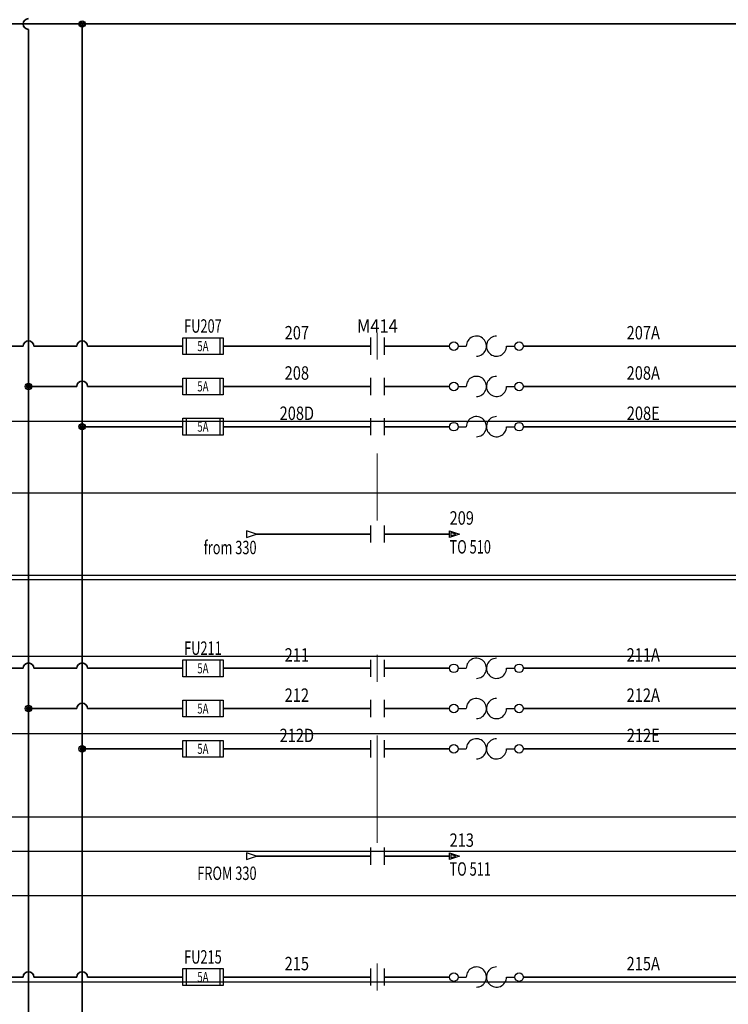
# Model space of a CAD drawing. Extents: x 0 to 33.5, y 0 to 22.4.
# Tile 3 of 8: x 6.7 to 13.3, y 8.5 to 17.7. Entities that reach past the tile are written whole.
import ezdxf
from ezdxf.enums import TextEntityAlignment as Align

# ---------------------------------------------------------------- set-up
doc = ezdxf.new("R2010")
doc.units = 0
doc.header["$MEASUREMENT"] = 0
for name, color, linetype, lineweight in [('A-ANNO-DIMS', 2, 'Continuous', 18), ('LINK', 9, 'Continuous', 18), ('MISC', 7, 'Continuous', 13), ('SYMS', 7, 'Continuous', 25), ('WIRENO', 72, 'Continuous', 18), ('WIRES', 7, 'Continuous', 35)]:
    doc.layers.add(name, color=color, linetype=linetype, lineweight=lineweight)
for name, color, linetype in [('DESC', 150, 'Continuous'), ('TAGS', 150, 'Continuous'), ('WIREREF', 52, 'Continuous'), ('XREF', 7, 'Continuous')]:
    doc.layers.add(name, color=color, linetype=linetype)
doc.styles.add('WD', font='romans.shx')
doc.dimstyles.get("Standard").update_dxf_attribs({"dimtxt": 0.18, "dimasz": 0.18, "dimexe": 0.18, "dimexo": 0.0625, "dimgap": 0.09, "dimtad": 0, "dimtih": 1, "dimtoh": 1, "dimdec": 4, "dimzin": 0, "dimdsep": 46, "dimtxsty": 'Standard', "dimcen": 0.09, "dimadec": 0, "dimazin": 0, "dimtfac": 1, "dimtdec": 4, "dimtofl": 0, "dimtmove": 0, "dimatfit": 3, "dimfxl": 1, "dimtolj": 1, "dimtzin": 0, "dimarcsym": 0})

# ---------------------------------------------------------------- blocks, each defined once
blk = doc.blocks.new('WDDOT')
for radius in [0.03, 0.0187, 0.00929]:
    blk.add_circle((0, 0), radius)
blk = doc.blocks.new('HFU1')
for p, q in [((-0.1875, -0.0781), (-0.1875, 0.0781)), ((-0.1875, 0.0781), (0.1875, 0.0781)), ((-0.1562, 0.0781), (-0.1562, -0.0781)), ((0.1562, 0.0781), (0.1562, -0.0781)), ((0.1875, 0.0781), (0.1875, -0.0781)), ((0.1875, -0.0781), (-0.1875, -0.0781))]:
    blk.add_line(p, q)
at = {"style": 'WD', "width": 0.7}
for tag, p in [('INST', (0, 0.4219)), ('LOC', (0, 0.2656)), ('TAG1', (0, 0.125))]:
    blk.add_attdef(tag, text='', height=0.125, dxfattribs=at).set_placement(p, align=Align.CENTER)
at = {"style": 'WD', "flags": 9}
for tag, p in [('ASSYCODE', (0.1569, 0.2509)), ('MFG', (0.1564, 0.0827)), ('CAT', (0.1564, 0.1022))]:
    blk.add_attdef(tag, text='', height=0.01, dxfattribs=at).set_placement(p, align=Align.CENTER)
at = {"style": 'WD'}
for tag, p in [('X2LINK', (0, 0.1094)), ('X8LINK', (0, -0.1094))]:
    blk.add_attdef(tag, p, '', height=0.01, dxfattribs=at)
for tag, p, height, flags in [('FAMILY', (0.1292, 0.1076), 0.01, 9), ('X4TERM01', (-0.1875, 0), 0.0109, 1), ('X1TERM02', (0.1875, 0), 0.0109, 1)]:
    blk.add_attdef(tag, p, '', height=height, dxfattribs=dict(at, flags=flags))
at = {"style": 'WD', "width": 0.7}
blk.add_attdef('RATING1', text='', height=0.0938, dxfattribs=at).set_placement((0, 0), align=Align.MIDDLE_CENTER)
at = {"style": 'WD', "width": 0.7, "flags": 8}
blk.add_attdef('TERM01', text='', height=0.1, dxfattribs=at).set_placement((-0.25, -0.0158), align=Align.TOP_RIGHT)
blk.add_attdef('TERM02', text='', height=0.1, dxfattribs=at).set_placement((0.25, -0.0158), align=Align.TOP_LEFT)
at = {"style": 'WD', "width": 0.7}
for tag, p in [('DESC1', (0.0469, -0.2344)), ('DESC2', (0.0469, -0.3906)), ('DESC3', (0.0469, -0.5469))]:
    blk.add_attdef(tag, text='', height=0.125, dxfattribs=at).set_placement(p, align=Align.MIDDLE_LEFT)
blk = doc.blocks.new('HCR21')
for p, q in [((-0.0625, 0.08), (-0.0625, -0.08)), ((0.0625, 0.08), (0.0625, -0.08))]:
    blk.add_line(p, q)
at = {"style": 'WD'}
for tag, width, p in [('INST', 0.7, (0, 0.4508)), ('LOC', 0.7, (0, 0.2812)), ('TAG2', 0.9, (0, 0.125)), ('XREF', 0.7, (0, -0.2975)), ('DESC1', 0.7, (0, -0.4495)), ('DESC2', 0.7, (0, -0.5968)), ('DESC3', 0.7, (0, -0.7442))]:
    blk.add_attdef(tag, text='', height=0.125, dxfattribs=dict(at, width=width)).set_placement(p, align=Align.CENTER)
for tag, p in [('X2LINK', (0, 0.125)), ('X8LINK', (0, -0.125))]:
    blk.add_attdef(tag, p, '', height=0.01, dxfattribs=at)
for tag, p, height, flags in [('X4TERM01', (-0.0625, 0), 0.0125, 1), ('X1TERM02', (0.0625, 0), 0.0125, 1), ('CONTACT', (0.0973, 0.0363), 0.01, 1), ('FAMILY', (0.0973, 0.0529), 0.01, 9)]:
    blk.add_attdef(tag, p, '', height=height, dxfattribs=dict(at, flags=flags))
at = {"style": 'WD', "flags": 8}
blk.add_attdef('TERM01', text='', height=0.125, dxfattribs=at).set_placement((-0.125, -0.0158), align=Align.TOP_RIGHT)
blk.add_attdef('TERM02', text='', height=0.125, dxfattribs=at).set_placement((0.125, -0.0158), align=Align.TOP_LEFT)
blk = doc.blocks.new('HOL1')
for p, q in [((-0.2637, 0), (-0.1875, 0)), ((0.1875, 0), (0.2637, 0))]:
    blk.add_line(p, q)
for centre in [(-0.3038, 0), (0.3038, 0)]:
    blk.add_circle(centre, 0.04)
for centre, start, end in [((-0.0938, 0), 270.00101, 180.00201), ((0.0938, 0), 90, 0.00104)]:
    blk.add_arc(centre, 0.0938, start, end)
at = {"style": 'WD', "width": 0.7}
for tag, p in [('INST', (0, 0.7946)), ('LOC', (0, 0.625)), ('DESC1', (0, 0.4688)), ('DESC2', (0, 0.3125)), ('RATING1', (0, -0.2656))]:
    blk.add_attdef(tag, text='', height=0.125, dxfattribs=at).set_placement(p, align=Align.CENTER)
at = {"style": 'WD'}
blk.add_attdef('TAG1', text='', height=0.125, dxfattribs=at).set_placement((0, 0.1562), align=Align.CENTER)
for tag, p in [('X2LINK', (0, 0.125)), ('X8LINK', (0, -0.125))]:
    blk.add_attdef(tag, p, '', height=0.01, dxfattribs=at)
for tag, p, height, flags in [('FAMILY', (0.2047, 0.1523), 0.01, 9), ('X4TERM01', (-0.3438, 0), 0.0125, 1), ('X1TERM02', (0.3438, 0), 0.0125, 1)]:
    blk.add_attdef(tag, p, '', height=height, dxfattribs=dict(at, flags=flags))
at = {"style": 'WD', "flags": 9}
for tag, p in [('MFG', (0.2278, 0.0887)), ('CAT', (0.2297, 0.1082)), ('ASSYCODE', (0.2188, 0.0625))]:
    blk.add_attdef(tag, text='', height=0.01, dxfattribs=at).set_placement(p, align=Align.CENTER)
at = {"style": 'WD', "flags": 8}
blk.add_attdef('TERM01', text='', height=0.125, dxfattribs=at).set_placement((-0.4062, -0.0314), align=Align.TOP_RIGHT)
blk.add_attdef('TERM02', text='', height=0.125, dxfattribs=at).set_placement((0.4062, -0.0314), align=Align.TOP_LEFT)
blk = doc.blocks.new('HA1S1')
for points in [[(0, 0), (0, 0.0312), (0.0938, 0), (0, -0.0312), (0, 0)], [(0.0106, 0.0156), (0.0106, -0.0156), (0.0575, 0), (0.0106, 0.0156)]]:
    blk.add_lwpolyline(points)
at = {"style": 'WD', "width": 0.8, "flags": 8}
blk.add_attdef('WIRENO', (0, 0.0875), '', height=0.125, dxfattribs=at)
at = {"style": 'WD', "flags": 1}
for tag, p in [('SIGCODE', (-0.0195, 0.0466)), ('X4TERM01', (0, 0))]:
    blk.add_attdef(tag, p, '', height=0.01, dxfattribs=at)
at = {"style": 'WD', "width": 0.7}
for tag, p in [('XREF', (0, -0.1812)), ('DESC1', (0, -0.3563))]:
    blk.add_attdef(tag, p, '', height=0.125, dxfattribs=at)
blk = doc.blocks.new('HA1D3')
blk.add_lwpolyline([(-0.0938, 0), (-0.0938, -0.0312), (0, 0), (-0.0938, 0.0312), (-0.0938, 0)])
at = {"style": 'WD', "width": 0.8, "flags": 8}
blk.add_attdef('WIRENO', text='', height=0.125, dxfattribs=at).set_placement((0, 0.0938), align=Align.RIGHT)
at = {"style": 'WD', "flags": 1}
blk.add_attdef('SIGCODE', text='', height=0.01, dxfattribs=at).set_placement((-0.0195, 0.0466), align=Align.RIGHT)
blk.add_attdef('X1TERM01', (0, 0), '', height=0.01, dxfattribs=at)
at = {"style": 'WD', "width": 0.7}
for tag, p in [('XREF', (0, -0.1875)), ('DESC1', (0, -0.375))]:
    blk.add_attdef(tag, text='', height=0.125, dxfattribs=at).set_placement(p, align=Align.RIGHT)
blk = doc.blocks.new('WD_WNH')
at = {"style": 'WD', "width": 0.8}
blk.add_attdef('WIRENO', text='', height=0.125, dxfattribs=at).set_placement((0, 0.0625), align=Align.CENTER)
at = {"style": 'WD', "flags": 1}
for tag, p in [('W01USER', (0, 0.0781)), ('W02USER', (0, 0.0703)), ('W03USER', (0, 0.0625)), ('W04USER', (0, 0.0547)), ('W05USER', (0, 0.0469)), ('W06USER', (0, 0.0391)), ('W07USER', (0, 0.0312)), ('W08USER', (0, 0.0234)), ('W09USER', (0, 0.0156)), ('W10USER', (0, 0.0078))]:
    blk.add_attdef(tag, text='', height=0.005, dxfattribs=at).set_placement(p, align=Align.CENTER)
blk = doc.blocks.new('*D46')
at = {"layer": 'A-ANNO-DIMS', "color": 0, "lineweight": -2, "transparency": 16777216}
for p, q in [((13.6523, 13.9244), (1.48, 13.9244)), ((1.66, 13.7444), (1.66, 13.3662)), ((1.66, 12.628), (1.66, 13.0062)), ((13.6816, 12.448), (1.48, 12.448))]:
    blk.add_line(p, q, dxfattribs=at)
at = {"layer": 'A-ANNO-DIMS', "color": 0, "transparency": 16777216}
for points in [[(1.63, 13.7444), (1.69, 13.7444), (1.66, 13.9244)], [(1.63, 12.628), (1.69, 12.628), (1.66, 12.448)]]:
    blk.add_solid(points, dxfattribs=at)
at = {"layer": 'Defpoints', "color": 0, "transparency": 16777216}
for p in [(13.7148, 13.9244), (1.66, 12.448), (13.7441, 12.448)]:
    blk.add_point(p, dxfattribs=at)
at = {"layer": 'A-ANNO-DIMS', "color": 0, "transparency": 16777216, "insert": (1.66, 13.1862), "char_height": 0.18, "attachment_point": 5}
blk.add_mtext('\\A1;1.48', dxfattribs=at)
blk = doc.blocks.new('*D47')
at = {"layer": 'A-ANNO-DIMS', "color": 0, "lineweight": -2, "transparency": 16777216}
for p, q in [((13.627211, 10.238995), (1.48, 10.238995)), ((1.66, 10.058995), (1.66, 9.686874)), ((13.627211, 9.506874), (1.48, 9.506874)), ((1.66, 9.506874), (1.66, 9.326874)), ((1.66, 9.326874), (1.48, 9.326874))]:
    blk.add_line(p, q, dxfattribs=at)
at = {"layer": 'A-ANNO-DIMS', "color": 0, "transparency": 16777216}
for points in [[(1.63, 10.058995), (1.69, 10.058995), (1.66, 10.238995)], [(1.63, 9.686874), (1.69, 9.686874), (1.66, 9.506874)]]:
    blk.add_solid(points, dxfattribs=at)
at = {"layer": 'Defpoints', "color": 0, "transparency": 16777216}
for p in [(13.689711, 10.238995), (1.66, 9.506874), (13.689711, 9.506874)]:
    blk.add_point(p, dxfattribs=at)
at = {"layer": 'A-ANNO-DIMS', "color": 0, "transparency": 16777216, "insert": (1.135, 9.326874), "char_height": 0.18, "attachment_point": 5}
blk.add_mtext('\\A1;0.73', dxfattribs=at)
blk = doc.blocks.new('*D56')
at = {"layer": 'A-ANNO-DIMS', "color": 0, "lineweight": -2, "transparency": 16777216}
for p, q in [((29.389766, 13.255775), (1.48, 13.255775)), ((1.66, 13.075775), (1.66, 12.669774)), ((29.4322, 12.489774), (1.48, 12.489774)), ((1.66, 12.489774), (1.66, 12.309774)), ((1.66, 12.309774), (1.48, 12.309774))]:
    blk.add_line(p, q, dxfattribs=at)
at = {"layer": 'A-ANNO-DIMS', "color": 0, "transparency": 16777216}
for points in [[(1.63, 13.075775), (1.69, 13.075775), (1.66, 13.255775)], [(1.63, 12.669774), (1.69, 12.669774), (1.66, 12.489774)]]:
    blk.add_solid(points, dxfattribs=at)
at = {"layer": 'Defpoints', "color": 0, "transparency": 16777216}
for p in [(29.452266, 13.255775), (1.66, 12.489774), (29.4947, 12.489774)]:
    blk.add_point(p, dxfattribs=at)
at = {"layer": 'A-ANNO-DIMS', "color": 0, "transparency": 16777216, "insert": (1.045, 12.309774), "char_height": 0.18, "attachment_point": 5}
blk.add_mtext('\\A1;0.766', dxfattribs=at)
blk = doc.blocks.new('*D57')
at = {"layer": 'A-ANNO-DIMS', "color": 0, "lineweight": -2, "transparency": 16777216}
for p, q in [((29.4322, 12.489774), (1.48, 12.489774)), ((1.66, 12.309774), (1.66, 11.913516)), ((29.435818, 11.733516), (1.48, 11.733516)), ((1.66, 11.733516), (1.66, 11.553516)), ((1.66, 11.553516), (1.48, 11.553516))]:
    blk.add_line(p, q, dxfattribs=at)
at = {"layer": 'A-ANNO-DIMS', "color": 0, "transparency": 16777216}
for points in [[(1.63, 12.309774), (1.69, 12.309774), (1.66, 12.489774)], [(1.63, 11.913516), (1.69, 11.913516), (1.66, 11.733516)]]:
    blk.add_solid(points, dxfattribs=at)
at = {"layer": 'Defpoints', "color": 0, "transparency": 16777216}
for p in [(29.4947, 12.489774), (1.66, 11.733516), (29.498318, 11.733516)]:
    blk.add_point(p, dxfattribs=at)
at = {"layer": 'A-ANNO-DIMS', "color": 0, "transparency": 16777216, "insert": (1.135, 11.553516), "char_height": 0.18, "attachment_point": 5}
blk.add_mtext('\\A1;0.76', dxfattribs=at)
blk = doc.blocks.new('*D58')
at = {"layer": 'A-ANNO-DIMS', "color": 0, "lineweight": -2, "transparency": 16777216}
for p, q in [((29.435818, 11.733516), (1.48, 11.733516)), ((1.66, 11.553516), (1.66, 11.194575)), ((29.438773, 11.014575), (1.48, 11.014575)), ((1.66, 11.014575), (1.66, 10.834575)), ((1.66, 10.834575), (1.48, 10.834575))]:
    blk.add_line(p, q, dxfattribs=at)
at = {"layer": 'A-ANNO-DIMS', "color": 0, "transparency": 16777216}
for points in [[(1.63, 11.553516), (1.69, 11.553516), (1.66, 11.733516)], [(1.63, 11.194575), (1.69, 11.194575), (1.66, 11.014575)]]:
    blk.add_solid(points, dxfattribs=at)
at = {"layer": 'Defpoints', "color": 0, "transparency": 16777216}
for p in [(29.498318, 11.733516), (1.66, 11.014575), (29.501273, 11.014575)]:
    blk.add_point(p, dxfattribs=at)
at = {"layer": 'A-ANNO-DIMS', "color": 0, "transparency": 16777216, "insert": (1.075, 10.834575), "char_height": 0.18, "attachment_point": 5}
blk.add_mtext('\\A1;0.719', dxfattribs=at)
blk = doc.blocks.new('*D59')
at = {"layer": 'A-ANNO-DIMS', "color": 0, "lineweight": -2, "transparency": 16777216}
for p, q in [((29.438773, 11.014575), (1.48, 11.014575)), ((1.66, 10.834575), (1.66, 10.646575)), ((1.66, 10.098575), (1.66, 10.286575)), ((29.435818, 9.918575), (1.48, 9.918575))]:
    blk.add_line(p, q, dxfattribs=at)
at = {"layer": 'A-ANNO-DIMS', "color": 0, "transparency": 16777216}
for points in [[(1.63, 10.834575), (1.69, 10.834575), (1.66, 11.014575)], [(1.63, 10.098575), (1.69, 10.098575), (1.66, 9.918575)]]:
    blk.add_solid(points, dxfattribs=at)
at = {"layer": 'Defpoints', "color": 0, "transparency": 16777216}
for p in [(29.501273, 11.014575), (1.66, 9.918575), (29.498318, 9.918575)]:
    blk.add_point(p, dxfattribs=at)
at = {"layer": 'A-ANNO-DIMS', "color": 0, "transparency": 16777216, "insert": (1.66, 10.466575), "char_height": 0.18, "attachment_point": 5}
blk.add_mtext('\\A1;1.096', dxfattribs=at)
blk = doc.blocks.new('*D60')
at = {"layer": 'A-ANNO-DIMS', "color": 0, "lineweight": -2, "transparency": 16777216}
for p, q in [((29.435818, 9.918575), (1.48, 9.918575)), ((1.66, 9.738575), (1.66, 9.490438)), ((1.66, 8.882301), (1.66, 9.130438)), ((29.4322, 8.702301), (1.48, 8.702301))]:
    blk.add_line(p, q, dxfattribs=at)
at = {"layer": 'A-ANNO-DIMS', "color": 0, "transparency": 16777216}
for points in [[(1.63, 9.738575), (1.69, 9.738575), (1.66, 9.918575)], [(1.63, 8.882301), (1.69, 8.882301), (1.66, 8.702301)]]:
    blk.add_solid(points, dxfattribs=at)
at = {"layer": 'Defpoints', "color": 0, "transparency": 16777216}
for p in [(29.498318, 9.918575), (1.66, 8.702301), (29.4947, 8.702301)]:
    blk.add_point(p, dxfattribs=at)
at = {"layer": 'A-ANNO-DIMS', "color": 0, "transparency": 16777216, "insert": (1.66, 9.310438), "char_height": 0.18, "attachment_point": 5}
blk.add_mtext('\\A1;1.22', dxfattribs=at)
blk = doc.blocks.new('*D61')
at = {"layer": 'A-ANNO-DIMS', "color": 0, "lineweight": -2, "transparency": 16777216}
for p, q in [((23.0885, 18.3786), (1.48, 18.3786)), ((1.66, 18.1986), (1.66, 15.9972)), ((1.66, 13.4358), (1.66, 15.6372)), ((20.8383, 13.2558), (1.48, 13.2558))]:
    blk.add_line(p, q, dxfattribs=at)
at = {"layer": 'A-ANNO-DIMS', "color": 0, "transparency": 16777216}
for points in [[(1.63, 18.1986), (1.69, 18.1986), (1.66, 18.3786)], [(1.63, 13.4358), (1.69, 13.4358), (1.66, 13.2558)]]:
    blk.add_solid(points, dxfattribs=at)
at = {"layer": 'Defpoints', "color": 0, "transparency": 16777216}
for p in [(23.151, 18.3786), (1.66, 13.2558), (20.9008, 13.2558)]:
    blk.add_point(p, dxfattribs=at)
at = {"layer": 'A-ANNO-DIMS', "color": 0, "transparency": 16777216, "insert": (1.66, 15.8172), "char_height": 0.18, "attachment_point": 5}
blk.add_mtext('\\A1;5.123', dxfattribs=at)

msp = doc.modelspace()

# ---------------------------------------------------------------- linework, layer by layer
at = {"layer": 'LINK'}
for points in [[(10, 14.5), (10, 14.75)], [(10, 11.5), (10, 11.75)], [(10, 10.625), (10, 11)], [(10, 8.625), (10, 8.875)]]:
    msp.add_lwpolyline(points, dxfattribs=at)
at = {"layer": 'LINK', "ltscale": 0.5}
for points in [[(10, 13.625), (10, 13)], [(10, 10.75), (10, 10)]]:
    msp.add_lwpolyline(points, dxfattribs=at)
at = {"layer": 'WIRES'}
for p, q in [((5.1875, 17.625), (30.0939, 17.625)), ((7.25, 17.625), (7.25, 7.875)), ((6.75, 17.575), (6.75, 8.25)), ((6.25, 14.625), (6.7, 14.625)), ((6.8, 14.625), (7.2, 14.625)), ((7.3, 14.625), (8.1875, 14.625)), ((8.5625, 14.625), (9.9375, 14.625)), ((10.0625, 14.625), (10.673, 14.625)), ((11.3605, 14.625), (13.5956, 14.625)), ((6.75, 14.25), (7.2, 14.25)), ((7.3, 14.25), (8.1875, 14.25)), ((8.5625, 14.25), (9.9375, 14.25)), ((10.0625, 14.25), (10.673, 14.25)), ((11.3605, 14.25), (13.5956, 14.25)), ((7.25, 13.875), (8.1875, 13.875)), ((8.5625, 13.875), (9.9375, 13.875)), ((10.0625, 13.875), (10.673, 13.875)), ((11.3605, 13.875), (13.5956, 13.875)), ((8.875, 12.875), (9.9375, 12.875)), ((10.0625, 12.875), (10.673, 12.875)), ((6.25, 11.625), (6.7, 11.625)), ((6.8, 11.625), (7.2, 11.625)), ((7.3, 11.625), (8.1875, 11.625)), ((8.5625, 11.625), (9.9375, 11.625)), ((10.0625, 11.625), (10.673, 11.625)), ((11.3605, 11.625), (13.5956, 11.625)), ((6.75, 11.25), (7.2, 11.25)), ((7.3, 11.25), (8.1875, 11.25)), ((8.5625, 11.25), (9.9375, 11.25)), ((10.0625, 11.25), (10.673, 11.25)), ((11.3605, 11.25), (13.5956, 11.25)), ((7.25, 10.875), (8.1875, 10.875)), ((8.5625, 10.875), (9.9375, 10.875)), ((10.0625, 10.875), (10.673, 10.875)), ((11.3605, 10.875), (13.5956, 10.875)), ((8.875, 9.875), (9.9375, 9.875)), ((10.0625, 9.875), (10.673, 9.875)), ((6.25, 8.75), (6.7, 8.75)), ((6.8, 8.75), (7.2, 8.75)), ((7.3, 8.75), (8.1875, 8.75)), ((8.5625, 8.75), (9.9375, 8.75)), ((10.0625, 8.75), (10.673, 8.75)), ((11.3605, 8.75), (13.5956, 8.75))]:
    msp.add_line(p, q, dxfattribs=at)
for centre, start, end in [((6.75, 17.625), 90, 270), ((6.75, 14.625), 0, 180), ((7.25, 14.625), 0, 180), ((7.25, 14.25), 360, 180), ((6.75, 11.625), 0, 180), ((7.25, 11.625), 0, 180), ((7.25, 11.25), 0, 180), ((6.75, 8.75), 0, 180), ((7.25, 8.75), 0, 180)]:
    msp.add_arc(centre, 0.05, start, end, dxfattribs=at)

# ---------------------------------------------------------------- block references
at = {"layer": 'SYMS'}
for name, p in [('WDDOT', (7.25, 17.625)), ('HCR21', (10, 14.625)), ('HOL1', (11.0167, 14.625)), ('HOL1', (11.0167, 14.25)), ('WDDOT', (6.75, 14.25)), ('HCR21', (10, 13.875)), ('HOL1', (11.0167, 13.875)), ('WDDOT', (7.25, 13.875)), ('HCR21', (10, 12.875)), ('HCR21', (10, 11.625)), ('HOL1', (11.0167, 11.625)), ('WDDOT', (6.75, 11.25)), ('HCR21', (10, 11.25)), ('HCR21', (10, 11.25)), ('HOL1', (11.0167, 11.25)), ('HCR21', (10, 10.875)), ('HOL1', (11.0167, 10.875)), ('WDDOT', (7.25, 10.875)), ('WDDOT', (7.25, 10.875)), ('HCR21', (10, 9.875)), ('HCR21', (10, 8.75)), ('HOL1', (11.0167, 8.75))]:
    msp.add_blockref(name, p, dxfattribs=at)
ref = msp.add_blockref('HFU1', (8.375, 14.625), dxfattribs=at)
ref.add_attrib('RATING1', '5A', dxfattribs={"layer": 'MISC', "height": 0.09375, "style": 'WD', "width": 0.7}).set_placement((8.375, 14.625), align=Align.MIDDLE_CENTER)
ref.add_attrib('TAG1', 'FU207', dxfattribs={"layer": 'TAGS', "height": 0.125, "style": 'WD', "width": 0.7}).set_placement((8.375, 14.75), align=Align.CENTER)
ref = msp.add_blockref('HCR21', (10, 14.25), dxfattribs=at)
ref.add_attrib('TAG2', 'M414', dxfattribs={"layer": 'TAGS', "height": 0.125, "style": 'WD', "width": 0.9}).set_placement((10, 14.75), align=Align.CENTER)
ref = msp.add_blockref('HFU1', (8.375, 14.25), dxfattribs=at)
ref.add_attrib('RATING1', '5A', dxfattribs={"layer": 'MISC', "height": 0.09375, "style": 'WD', "width": 0.7}).set_placement((8.375, 14.25), align=Align.MIDDLE_CENTER)
ref = msp.add_blockref('HFU1', (8.375, 13.875), dxfattribs=at)
ref.add_attrib('RATING1', '5A', dxfattribs={"layer": 'MISC', "height": 0.09375, "style": 'WD', "width": 0.7}).set_placement((8.375, 13.875), align=Align.MIDDLE_CENTER)
ref = msp.add_blockref('HA1S1', (10.673, 12.875), dxfattribs=at)
ref.add_attrib('DESC1', 'TO 510', (10.673, 12.6937), dxfattribs={"layer": 'DESC', "height": 0.125, "style": 'WD', "width": 0.7})
ref.add_attrib('WIRENO', '209', (10.673, 12.9625), dxfattribs={"layer": 'WIREREF', "height": 0.125, "style": 'WD', "width": 0.8, "flags": 8})
ref = msp.add_blockref('HA1D3', (8.875, 12.875), dxfattribs=at)
ref.add_attrib('XREF', 'from 330', dxfattribs={"layer": 'XREF', "height": 0.125, "style": 'WD', "width": 0.7}).set_placement((8.875, 12.6875), align=Align.RIGHT)
ref = msp.add_blockref('HFU1', (8.375, 11.625), dxfattribs=at)
ref.add_attrib('RATING1', '5A', dxfattribs={"layer": 'MISC', "height": 0.09375, "style": 'WD', "width": 0.7}).set_placement((8.375, 11.625), align=Align.MIDDLE_CENTER)
ref.add_attrib('TAG1', 'FU211', dxfattribs={"layer": 'TAGS', "height": 0.125, "style": 'WD', "width": 0.7}).set_placement((8.375, 11.75), align=Align.CENTER)
ref = msp.add_blockref('HFU1', (8.375, 11.25), dxfattribs=at)
ref.add_attrib('RATING1', '5A', dxfattribs={"layer": 'MISC', "height": 0.09375, "style": 'WD', "width": 0.7}).set_placement((8.375, 11.25), align=Align.MIDDLE_CENTER)
ref = msp.add_blockref('HFU1', (8.375, 10.875), dxfattribs=at)
ref.add_attrib('RATING1', '5A', dxfattribs={"layer": 'MISC', "height": 0.09375, "style": 'WD', "width": 0.7}).set_placement((8.375, 10.875), align=Align.MIDDLE_CENTER)
ref = msp.add_blockref('HA1S1', (10.673, 9.875), dxfattribs=at)
ref.add_attrib('DESC1', 'TO 511', (10.673, 9.6937), dxfattribs={"layer": 'DESC', "height": 0.125, "style": 'WD', "width": 0.7})
ref.add_attrib('WIRENO', '213', (10.673, 9.9625), dxfattribs={"layer": 'WIREREF', "height": 0.125, "style": 'WD', "width": 0.8, "flags": 8})
ref = msp.add_blockref('HA1D3', (8.875, 9.875), dxfattribs=at)
ref.add_attrib('DESC1', 'FROM 330', dxfattribs={"layer": 'DESC', "height": 0.125, "style": 'WD', "width": 0.7}).set_placement((8.875, 9.6539), align=Align.RIGHT)
ref = msp.add_blockref('HFU1', (8.375, 8.75), dxfattribs=at)
ref.add_attrib('RATING1', '5A', dxfattribs={"layer": 'MISC', "height": 0.09375, "style": 'WD', "width": 0.7}).set_placement((8.375, 8.75), align=Align.MIDDLE_CENTER)
ref.add_attrib('TAG1', 'FU215', dxfattribs={"layer": 'TAGS', "height": 0.125, "style": 'WD', "width": 0.7}).set_placement((8.375, 8.875), align=Align.CENTER)
at = {"layer": 'WIRENO'}
ref = msp.add_blockref('WD_WNH', (9.25, 14.625), dxfattribs=at)
ref.add_attrib('WIRENO', '207', dxfattribs={"linetype": 'Continuous', "height": 0.125, "style": 'WD', "width": 0.8}).set_placement((9.25, 14.6875), align=Align.CENTER)
ref = msp.add_blockref('WD_WNH', (12.478, 14.625), dxfattribs=at)
ref.add_attrib('WIRENO', '207A', dxfattribs={"linetype": 'Continuous', "height": 0.125, "style": 'WD', "width": 0.8}).set_placement((12.478, 14.6875), align=Align.CENTER)
ref = msp.add_blockref('WD_WNH', (9.25, 14.25), dxfattribs=at)
ref.add_attrib('WIRENO', '208', dxfattribs={"linetype": 'Continuous', "height": 0.125, "style": 'WD', "width": 0.8}).set_placement((9.25, 14.3125), align=Align.CENTER)
ref = msp.add_blockref('WD_WNH', (12.478, 14.25), dxfattribs=at)
ref.add_attrib('WIRENO', '208A', dxfattribs={"linetype": 'Continuous', "height": 0.125, "style": 'WD', "width": 0.8}).set_placement((12.478, 14.3125), align=Align.CENTER)
ref = msp.add_blockref('WD_WNH', (9.25, 13.875), dxfattribs=at)
ref.add_attrib('WIRENO', '208D', dxfattribs={"linetype": 'Continuous', "height": 0.125, "style": 'WD', "width": 0.8}).set_placement((9.25, 13.9375), align=Align.CENTER)
ref = msp.add_blockref('WD_WNH', (12.478, 13.875), dxfattribs=at)
ref.add_attrib('WIRENO', '208E', dxfattribs={"linetype": 'Continuous', "height": 0.125, "style": 'WD', "width": 0.8}).set_placement((12.478, 13.9375), align=Align.CENTER)
ref = msp.add_blockref('WD_WNH', (9.25, 11.625), dxfattribs=at)
ref.add_attrib('WIRENO', '211', dxfattribs={"linetype": 'Continuous', "height": 0.125, "style": 'WD', "width": 0.8}).set_placement((9.25, 11.6875), align=Align.CENTER)
ref = msp.add_blockref('WD_WNH', (12.478, 11.625), dxfattribs=at)
ref.add_attrib('WIRENO', '211A', dxfattribs={"linetype": 'Continuous', "height": 0.125, "style": 'WD', "width": 0.8}).set_placement((12.478, 11.6875), align=Align.CENTER)
ref = msp.add_blockref('WD_WNH', (9.25, 11.25), dxfattribs=at)
ref.add_attrib('WIRENO', '212', dxfattribs={"linetype": 'Continuous', "height": 0.125, "style": 'WD', "width": 0.8}).set_placement((9.25, 11.3125), align=Align.CENTER)
ref = msp.add_blockref('WD_WNH', (12.478, 11.25), dxfattribs=at)
ref.add_attrib('WIRENO', '212A', dxfattribs={"linetype": 'Continuous', "height": 0.125, "style": 'WD', "width": 0.8}).set_placement((12.478, 11.3125), align=Align.CENTER)
ref = msp.add_blockref('WD_WNH', (9.25, 10.875), dxfattribs=at)
ref.add_attrib('WIRENO', '212D', dxfattribs={"linetype": 'Continuous', "height": 0.125, "style": 'WD', "width": 0.8}).set_placement((9.25, 10.9375), align=Align.CENTER)
ref = msp.add_blockref('WD_WNH', (12.478, 10.875), dxfattribs=at)
ref.add_attrib('WIRENO', '212E', dxfattribs={"linetype": 'Continuous', "height": 0.125, "style": 'WD', "width": 0.8}).set_placement((12.478, 10.9375), align=Align.CENTER)
ref = msp.add_blockref('WD_WNH', (9.25, 8.75), dxfattribs=at)
ref.add_attrib('WIRENO', '215', dxfattribs={"linetype": 'Continuous', "height": 0.125, "style": 'WD', "width": 0.8}).set_placement((9.25, 8.8125), align=Align.CENTER)
ref = msp.add_blockref('WD_WNH', (12.478, 8.75), dxfattribs=at)
ref.add_attrib('WIRENO', '215A', dxfattribs={"linetype": 'Continuous', "height": 0.125, "style": 'WD', "width": 0.8}).set_placement((12.478, 8.8125), align=Align.CENTER)

# ---------------------------------------------------------------- dimensions: what is measured, and where the dimension line sits
at = {"layer": 'A-ANNO-DIMS'}
for base, p1, p2, override, picture, middle in [((1.66, 13.2558), (23.151, 18.3786), (20.9008, 13.2558), {"dimdec": 3, "dimlfac": 1, "dimrnd": 0, "dimzin": 0, "dimdsep": 46, "dimlunit": 2}, '*D61', (1.66, 15.8172)), ((1.66, 12.448), (13.7148, 13.9244), (13.7441, 12.448), {"dimdec": 2, "dimlfac": 1, "dimrnd": 0, "dimzin": 0, "dimdsep": 46, "dimlunit": 2}, '*D46', (1.66, 13.1862)), ((1.66, 12.4898), (29.4523, 13.2558), (29.4947, 12.4898), {"dimdec": 3, "dimlfac": 1, "dimrnd": 0, "dimzin": 0, "dimdsep": 46, "dimlunit": 2}, '*D56', (1.045, 12.3098)), ((1.66, 11.7335), (29.4947, 12.4898), (29.4983, 11.7335), {"dimdec": 2, "dimlfac": 1, "dimrnd": 0, "dimzin": 0, "dimdsep": 46, "dimlunit": 2}, '*D57', (1.135, 11.5535)), ((1.66, 11.0146), (29.4983, 11.7335), (29.5013, 11.0146), {"dimdec": 3, "dimlfac": 1, "dimrnd": 0, "dimzin": 0, "dimdsep": 46, "dimlunit": 2}, '*D58', (1.075, 10.8346)), ((1.66, 9.9186), (29.5013, 11.0146), (29.4983, 9.9186), {"dimdec": 3, "dimlfac": 1, "dimrnd": 0, "dimzin": 0, "dimdsep": 46, "dimlunit": 2}, '*D59', (1.66, 10.4666)), ((1.66, 9.5069), (13.6897, 10.239), (13.6897, 9.5069), {"dimdec": 2, "dimlfac": 1, "dimrnd": 0, "dimzin": 0, "dimdsep": 46, "dimlunit": 2}, '*D47', (1.135, 9.3269)), ((1.66, 8.7023), (29.4983, 9.9186), (29.4947, 8.7023), {"dimdec": 2, "dimlfac": 1, "dimrnd": 0, "dimzin": 0, "dimdsep": 46, "dimlunit": 2}, '*D60', (1.66, 9.3104))]:
    dim = msp.add_linear_dim(base=base, p1=p1, p2=p2, angle=90, dimstyle='Standard', override=override, dxfattribs=at)
    dim.commit()
    dim.dimension.update_dxf_attribs({"geometry": picture, "text_midpoint": middle})

doc.saveas('drawing.dxf')
